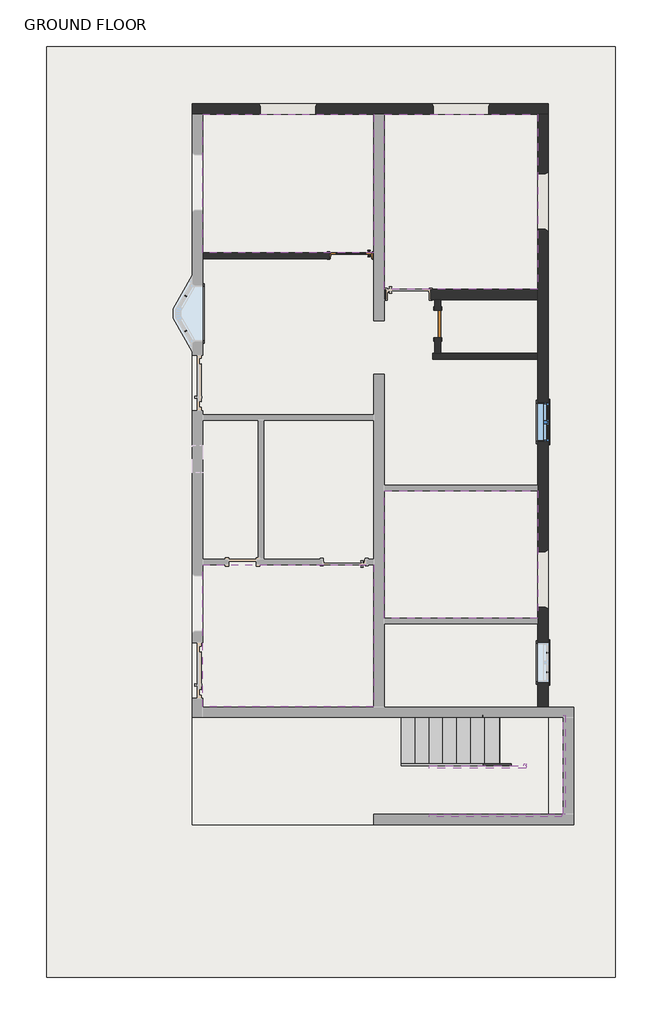
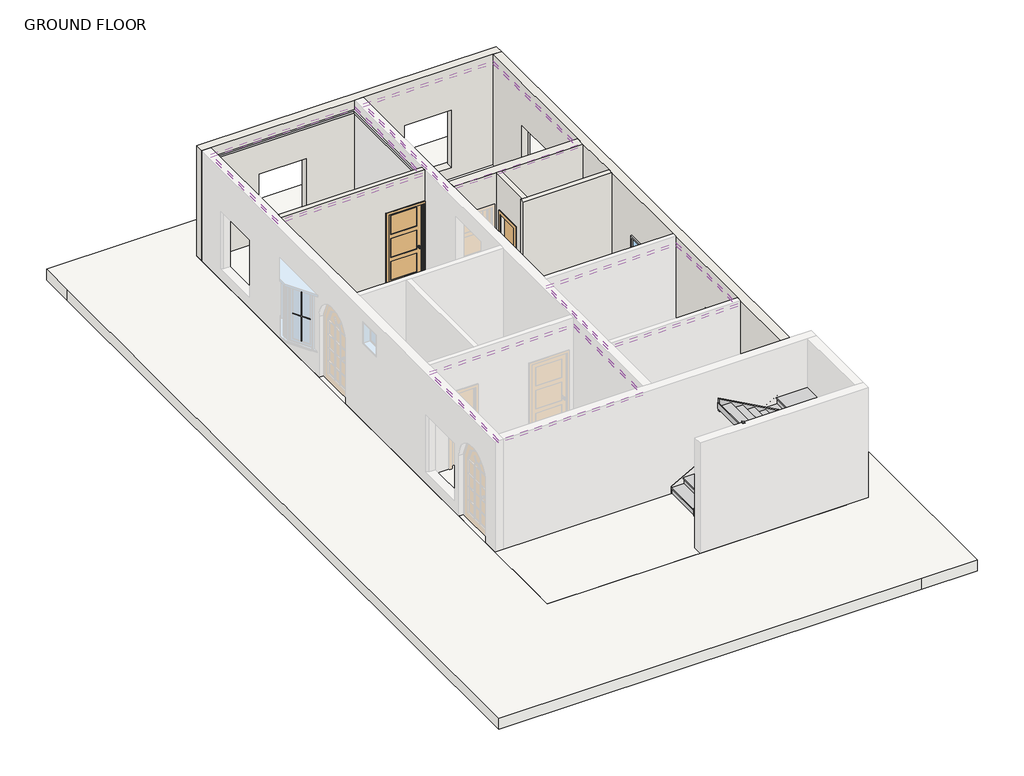
# One storey, part 2 of 2: 12 proxies, 8 coverings, 6 members, 6 walls, 2 doors, 2 slabs, 1 stair flight, 1 window.
"""IFC4 building model written with IfcOpenShell, lengths in millimetres."""

from ifc_helpers import new_model, si_unit, frame, origin, origin_with_axes, place, context, project, spatial, polyline, outline, extrude, faceted_brep, transform, mapped, element, save
from components import generic_models_1_generic_models_1_a1fc493f, muntin_pattern_2x2_muntin_pattern_2x2_75bf01dd, muntin_pattern_2x2_muntin_pattern_2x2_32baafd4, muntin_pattern_2x2_muntin_pattern_2x2_b3fe6957, muntin_pattern_2x2_muntin_pattern_2x2_3e0ecaf2, trim_window_exterior_flat_with_sill_41619996, trim_window_interior_flat_picture_frame_1060724f, trim_window_interior_flat_picture_frame_51c85655, door_b31adefa, single_flush_bathroom_flush_door_2_x_7_025d1c86, stair_flight_68498a3f, window_339605e1

model = new_model("IFC4")

# Units and contexts
model_context = context("Model", 3, world=origin())
ifc_project = project(units=[si_unit("LENGTHUNIT", "METRE", prefix="MILLI")], contexts=[model_context])

# Site, building, storey
site = spatial("IfcSite", under=ifc_project)
building = spatial("IfcBuilding", under=site)
storey = spatial("IfcBuildingStorey", under=building, Name="GROUND FLOOR", Elevation=304.8)

# Proxies
placement = place(None, origin())
generic_models_1_generic_models_1_shape = generic_models_1_generic_models_1_a1fc493f(model_context)
element("IfcBuildingElementProxy", 1, Name="Generic Models 1 : Generic Models 1", ObjectType="Generic Models 1 : Generic Models 1", at=placement, inside=storey, context=model_context, shape_type="MappedRepresentation", body=[
    mapped(generic_models_1_generic_models_1_shape, transform((0.0, 0.0, 0.0), x_axis=(1.0, 0.0, 0.0), y_axis=(0.0, 1.0, 0.0), z_axis=(0.0, 0.0, 1.0))),
])
muntin_pattern_2x2_muntin_pattern_2x2_shape = muntin_pattern_2x2_muntin_pattern_2x2_75bf01dd(model_context)
element("IfcBuildingElementProxy", 2, Name="Muntin Pattern_2x2 : Muntin Pattern_2x2", ObjectType="Muntin Pattern_2x2 : Muntin Pattern_2x2", at=placement, inside=storey, context=model_context, shape_type="MappedRepresentation", body=[
    mapped(muntin_pattern_2x2_muntin_pattern_2x2_shape, transform((-17494.1197687, 6617.7003691, 1035.05), x_axis=(-0.49999999999999245, 0.866025403784443, 0.0), y_axis=(-0.866025403784443, -0.49999999999999245, 0.0), z_axis=(0.0, 0.0, 1.0))),
])
muntin_pattern_2x2_muntin_pattern_2x2_2_shape = muntin_pattern_2x2_muntin_pattern_2x2_32baafd4(model_context)
element("IfcBuildingElementProxy", 3, Name="Muntin Pattern_2x2 : Muntin Pattern_2x2", ObjectType="Muntin Pattern_2x2 : Muntin Pattern_2x2", at=placement, inside=storey, context=model_context, shape_type="MappedRepresentation", body=[
    mapped(muntin_pattern_2x2_muntin_pattern_2x2_2_shape, transform((-17494.1197687, 7380.2948055, 1035.05), x_axis=(-0.4999999999999952, -0.8660254037844415, 0.0), y_axis=(0.8660254037844415, -0.4999999999999952, 0.0), z_axis=(0.0, 0.0, 1.0))),
])
muntin_pattern_2x2_muntin_pattern_2x2_3_shape = muntin_pattern_2x2_muntin_pattern_2x2_b3fe6957(model_context)
element("IfcBuildingElementProxy", 4, Name="Muntin Pattern_2x2 : Muntin Pattern_2x2", ObjectType="Muntin Pattern_2x2 : Muntin Pattern_2x2", at=placement, inside=storey, context=model_context, shape_type="MappedRepresentation", body=[
    mapped(muntin_pattern_2x2_muntin_pattern_2x2_3_shape, transform((-9539.4686606, -457.4899127, 1289.05), x_axis=(0.0, -1.0, 0.0), y_axis=(1.0, 0.0, 0.0), z_axis=(0.0, 0.0, 1.0))),
])
element("IfcBuildingElementProxy", 5, Name="Muntin Pattern_2x2 : Muntin Pattern_2x2", ObjectType="Muntin Pattern_2x2 : Muntin Pattern_2x2", at=placement, inside=storey, context=model_context, shape_type="MappedRepresentation", body=[
    mapped(muntin_pattern_2x2_muntin_pattern_2x2_3_shape, transform((-9539.4686606, 4825.7100873, 1289.05), x_axis=(0.0, -1.0, 0.0), y_axis=(1.0, 0.0, 0.0), z_axis=(0.0, 0.0, 1.0))),
])
muntin_pattern_2x2_muntin_pattern_2x2_4_shape = muntin_pattern_2x2_muntin_pattern_2x2_3e0ecaf2(model_context)
element("IfcBuildingElementProxy", 6, Name="Muntin Pattern_2x2 : Muntin Pattern_2x2", ObjectType="Muntin Pattern_2x2 : Muntin Pattern_2x2", at=placement, inside=storey, context=model_context, shape_type="MappedRepresentation", body=[
    mapped(muntin_pattern_2x2_muntin_pattern_2x2_4_shape, transform((-9539.4686606, -886.1149127, 1289.05), x_axis=(0.0, 1.0, 0.0), y_axis=(-1.0, 0.0, 0.0), z_axis=(0.0, 0.0, 1.0))),
])
element("IfcBuildingElementProxy", 7, Name="Muntin Pattern_2x2 : Muntin Pattern_2x2", ObjectType="Muntin Pattern_2x2 : Muntin Pattern_2x2", at=placement, inside=storey, context=model_context, shape_type="MappedRepresentation", body=[
    mapped(muntin_pattern_2x2_muntin_pattern_2x2_4_shape, transform((-9539.4686606, 4397.0850873, 1289.05), x_axis=(0.0, 1.0, 0.0), y_axis=(-1.0, 0.0, 0.0), z_axis=(0.0, 0.0, 1.0))),
])
trim_window_exterior_flat_with_sill_shape = trim_window_exterior_flat_with_sill_41619996(model_context)
element("IfcBuildingElementProxy", 8, Name="Trim-Window-Exterior-Flat : with Sill", ObjectType="Trim-Window-Exterior-Flat : with Sill", at=placement, inside=storey, context=model_context, shape_type="MappedRepresentation", body=[
    mapped(trim_window_exterior_flat_with_sill_shape, transform((-9529.9436606, -671.8024127, 2133.6), x_axis=(0.0, 1.0, 0.0), y_axis=(0.0, 0.0, 1.0), z_axis=(1.0, 0.0, 0.0))),
])
element("IfcBuildingElementProxy", 9, Name="Trim-Window-Exterior-Flat : with Sill", ObjectType="Trim-Window-Exterior-Flat : with Sill", at=placement, inside=storey, context=model_context, shape_type="MappedRepresentation", body=[
    mapped(trim_window_exterior_flat_with_sill_shape, transform((-9529.9436606, 4611.3975873, 2133.6), x_axis=(0.0, 1.0, 0.0), y_axis=(0.0, 0.0, 1.0), z_axis=(1.0, 0.0, 0.0))),
])
trim_window_interior_flat_picture_frame_shape = trim_window_interior_flat_picture_frame_1060724f(model_context)
element("IfcBuildingElementProxy", 10, Name="Trim-Window-Interior-Flat : Picture Frame", ObjectType="Trim-Window-Interior-Flat : Picture Frame", at=placement, inside=storey, context=model_context, shape_type="MappedRepresentation", body=[
    mapped(trim_window_interior_flat_picture_frame_shape, transform((-17124.5436606, 6998.9975873, 2489.2), x_axis=(0.0, 1.0, 0.0), y_axis=(0.0, 0.0, 1.0), z_axis=(1.0, 0.0, 0.0))),
])
trim_window_interior_flat_picture_frame_2_shape = trim_window_interior_flat_picture_frame_51c85655(model_context)
element("IfcBuildingElementProxy", 11, Name="Trim-Window-Interior-Flat : Picture Frame", ObjectType="Trim-Window-Interior-Flat : Picture Frame", at=placement, inside=storey, context=model_context, shape_type="MappedRepresentation", body=[
    mapped(trim_window_interior_flat_picture_frame_2_shape, transform((-9758.5436606, -671.8024127, 2133.6), x_axis=(0.0, -1.0, 0.0), y_axis=(0.0, 0.0, 1.0), z_axis=(-1.0, 0.0, 0.0))),
])
element("IfcBuildingElementProxy", 12, Name="Trim-Window-Interior-Flat : Picture Frame", ObjectType="Trim-Window-Interior-Flat : Picture Frame", at=placement, inside=storey, context=model_context, shape_type="MappedRepresentation", body=[
    mapped(trim_window_interior_flat_picture_frame_2_shape, transform((-9758.5436606, 4611.3975873, 2133.6), x_axis=(0.0, -1.0, 0.0), y_axis=(0.0, 0.0, 1.0), z_axis=(-1.0, 0.0, 0.0))),
])

# Coverings
element("IfcCovering", 13, ObjectType="ceiling", at=placement, inside=storey, context=model_context, shape_type="SweptSolid", body=[
    extrude(outline(polyline([(-17124.5436606, 8332.4975873), (-17124.5436606, 11380.4975873), (-13365.3436606, 11380.4975873), (-13365.3436606, 8332.4975873), (-17124.5436606, 8332.4975873)])), frame((0.0, 0.0, 3175.0), z_axis=(0.0, 0.0, 1.0), x_axis=(1.0, 0.0, 0.0)), (0.0, 0.0, 1.0), 107.95),
])
element("IfcCovering", 14, ObjectType="ceiling", at=placement, inside=storey, context=model_context, shape_type="SweptSolid", body=[
    extrude(outline(polyline([(-13365.3436606, 11380.4975873), (-13365.3436606, 8332.4975873), (-17124.5436606, 8332.4975873), (-17124.5436606, 11380.4975873), (-13365.3436606, 11380.4975873)]), holes=[polyline([(-13670.1436606, 11075.6975873), (-16819.7436606, 11075.6975873), (-16819.7436606, 8637.2975873), (-13670.1436606, 8637.2975873), (-13670.1436606, 11075.6975873)])]), frame((0.0, 0.0, 3098.8), z_axis=(0.0, 0.0, 1.0), x_axis=(1.0, 0.0, 0.0)), (0.0, 0.0, 1.0), 107.95),
    extrude(outline(polyline([(-14279.7436606, 10466.0975873), (-14279.7436606, 9246.8975873), (-16210.1436606, 9246.8975873), (-16210.1436606, 10466.0975873), (-14279.7436606, 10466.0975873)])), frame((0.0, 0.0, 3098.8), z_axis=(0.0, 0.0, 1.0), x_axis=(1.0, 0.0, 0.0)), (0.0, 0.0, 1.0), 107.95),
])
element("IfcCovering", 15, ObjectType="ceiling", at=placement, inside=storey, context=model_context, shape_type="SweptSolid", body=[
    extrude(outline(polyline([(-13136.7436606, 7532.3975873), (-13136.7436606, 11380.4975873), (-9758.5436606, 11380.4975873), (-9758.5436606, 7532.3975873), (-13136.7436606, 7532.3975873)])), frame((0.0, 0.0, 3175.0), z_axis=(0.0, 0.0, 1.0), x_axis=(1.0, 0.0, 0.0)), (0.0, 0.0, 1.0), 107.95),
])
element("IfcCovering", 16, ObjectType="ceiling", at=placement, inside=storey, context=model_context, shape_type="SweptSolid", body=[
    extrude(outline(polyline([(-9758.5436606, 11380.4975873), (-9758.5436606, 7532.3975873), (-13136.7436606, 7532.3975873), (-13136.7436606, 11380.4975873), (-9758.5436606, 11380.4975873)]), holes=[polyline([(-10063.3436606, 11075.6975873), (-12831.9436606, 11075.6975873), (-12831.9436606, 7837.1975873), (-10063.3436606, 7837.1975873), (-10063.3436606, 11075.6975873)])]), frame((0.0, 0.0, 3098.8), z_axis=(0.0, 0.0, 1.0), x_axis=(1.0, 0.0, 0.0)), (0.0, 0.0, 1.0), 107.95),
    extrude(outline(polyline([(-10672.9436606, 10466.0975873), (-10672.9436606, 8446.7975873), (-12222.3436606, 8446.7975873), (-12222.3436606, 10466.0975873), (-10672.9436606, 10466.0975873)])), frame((0.0, 0.0, 3098.8), z_axis=(0.0, 0.0, 1.0), x_axis=(1.0, 0.0, 0.0)), (0.0, 0.0, 1.0), 107.95),
])
element("IfcCovering", 17, ObjectType="ceiling", at=placement, inside=storey, context=model_context, shape_type="SweptSolid", body=[
    extrude(outline(polyline([(-13365.3436606, -1649.7024127), (-17124.5436606, -1649.7024127), (-17124.5436606, 1474.4975873), (-13365.3436606, 1474.4975873), (-13365.3436606, -1649.7024127)])), frame((0.0, 0.0, 3175.0), z_axis=(0.0, 0.0, 1.0), x_axis=(1.0, 0.0, 0.0)), (0.0, 0.0, 1.0), 107.95),
])
element("IfcCovering", 18, ObjectType="ceiling", at=placement, inside=storey, context=model_context, shape_type="SweptSolid", body=[
    extrude(outline(polyline([(-13365.3436606, 1474.4975873), (-13365.3436606, -1649.7024127), (-17124.5436606, -1649.7024127), (-17124.5436606, 1474.4975873), (-13365.3436606, 1474.4975873)]), holes=[polyline([(-13670.1436606, 1169.6975873), (-16819.7436606, 1169.6975873), (-16819.7436606, -1344.9024127), (-13670.1436606, -1344.9024127), (-13670.1436606, 1169.6975873)])]), frame((0.0, 0.0, 3098.8), z_axis=(0.0, 0.0, 1.0), x_axis=(1.0, 0.0, 0.0)), (0.0, 0.0, 1.0), 107.95),
    extrude(outline(polyline([(-14279.7436606, 560.0975873), (-14279.7436606, -735.3024127), (-16210.1436606, -735.3024127), (-16210.1436606, 560.0975873), (-14279.7436606, 560.0975873)])), frame((0.0, 0.0, 3098.8), z_axis=(0.0, 0.0, 1.0), x_axis=(1.0, 0.0, 0.0)), (0.0, 0.0, 1.0), 107.95),
])
element("IfcCovering", 19, ObjectType="ceiling", at=placement, inside=storey, context=model_context, shape_type="SweptSolid", body=[
    extrude(outline(polyline([(-9758.5436606, 3100.0975873), (-9758.5436606, 306.0975873), (-13136.7436606, 306.0975873), (-13136.7436606, 3100.0975873), (-9758.5436606, 3100.0975873)])), frame((0.0, 0.0, 3175.0), z_axis=(0.0, 0.0, 1.0), x_axis=(1.0, 0.0, 0.0)), (0.0, 0.0, 1.0), 107.95),
])
element("IfcCovering", 20, ObjectType="ceiling", at=placement, inside=storey, context=model_context, shape_type="SweptSolid", body=[
    extrude(outline(polyline([(-9758.5436606, 3100.0975873), (-9758.5436606, 306.0975873), (-13136.7436606, 306.0975873), (-13136.7436606, 3100.0975873), (-9758.5436606, 3100.0975873)]), holes=[polyline([(-10063.3436606, 2795.2975873), (-12831.9436606, 2795.2975873), (-12831.9436606, 610.8975873), (-10063.3436606, 610.8975873), (-10063.3436606, 2795.2975873)])]), frame((0.0, 0.0, 3098.8), z_axis=(0.0, 0.0, 1.0), x_axis=(1.0, 0.0, 0.0)), (0.0, 0.0, 1.0), 107.95),
    extrude(outline(polyline([(-10672.9436606, 2185.6975873), (-10672.9436606, 1220.4975873), (-12222.3436606, 1220.4975873), (-12222.3436606, 2185.6975873), (-10672.9436606, 2185.6975873)])), frame((0.0, 0.0, 3098.8), z_axis=(0.0, 0.0, 1.0), x_axis=(1.0, 0.0, 0.0)), (0.0, 0.0, 1.0), 107.95),
])

# Doors
door_shape = door_b31adefa(model_context)
element("IfcDoor", 21, ObjectType="Door-Interior-Single-3_Panel_Vert-Wood : 36\" x 84\"", at=placement, inside=storey, context=model_context, shape_type="MappedRepresentation", body=[
    mapped(door_shape, transform((-13860.6436606, 8272.1725873, 304.8), x_axis=(-1.0, 0.0, 0.0), y_axis=(0.0, -1.0, 0.0), z_axis=(0.0, 0.0, 1.0))),
])
single_flush_bathroom_flush_door_2_x_7_shape = single_flush_bathroom_flush_door_2_x_7_025d1c86(model_context)
element("IfcDoor", 22, ObjectType="Single-Flush : BATHROOM FLUSH DOOR 2' X 7'", at=placement, inside=storey, context=model_context, shape_type="MappedRepresentation", body=[
    mapped(single_flush_bathroom_flush_door_2_x_7_shape, transform((-11955.6436606, 6770.3975873, 304.8), x_axis=(0.0, -1.0, 0.0), y_axis=(1.0, 0.0, 0.0), z_axis=(0.0, 0.0, 1.0))),
])

# Members
element("IfcMember", 23, ObjectType="Stringer - 2\" Width", at=placement, inside=storey, context=model_context, shape_type="SweptSolid", body=[
    extrude(outline(polyline([(512.3983948, -12755.7436606), (304.8, -12755.7436606), (304.8, -12501.7991578), (2074.3333333, -9316.6391578), (2074.3333333, -9944.2607712), (512.3983948, -12755.7436606)])), frame((0.0, -1878.3024127, 0.0), z_axis=(0.0, 1.0, 0.0), x_axis=(0.0, 0.0, 1.0)), (0.0, 0.0, 1.0), 50.8),
])
element("IfcMember", 24, ObjectType="Stringer - 2\" Width", at=placement, inside=storey, context=model_context, shape_type="SweptSolid", body=[
    extrude(outline(polyline([(-9199.7436606, -1827.5024127), (-9148.9436606, -1827.5024127), (-9148.9436606, -4011.9024127), (-9199.7436606, -4011.9024127), (-9199.7436606, -1827.5024127)])), frame((0.0, 0.0, 1769.5333333), z_axis=(0.0, 0.0, 1.0), x_axis=(1.0, 0.0, 0.0)), (0.0, 0.0, 1.0), 304.8),
])
element("IfcMember", 25, ObjectType="Stringer - 2\" Width", at=placement, inside=storey, context=model_context, shape_type="SweptSolid", body=[
    extrude(outline(polyline([(1769.5333333, -9227.38655), (3391.0650614, -12146.1436606), (3042.3863873, -12146.1436606), (1769.5333333, -9855.0081634), (1769.5333333, -9227.38655)])), frame((0.0, -4062.7024127, 0.0), z_axis=(0.0, 1.0, 0.0), x_axis=(0.0, 0.0, 1.0)), (0.0, 0.0, 1.0), 50.8),
])
element("IfcMember", 26, ObjectType="Stringer - 2\" Width", at=placement, inside=storey, context=model_context, shape_type="SweptSolid", body=[
    extrude(outline(polyline([(512.3983948, -12755.7436606), (304.8, -12755.7436606), (304.8, -12501.7991578), (1659.4974984, -10063.3436606), (2008.1761726, -10063.3436606), (512.3983948, -12755.7436606)])), frame((0.0, -2945.1024127, 0.0), z_axis=(0.0, 1.0, 0.0), x_axis=(0.0, 0.0, 1.0)), (0.0, 0.0, 1.0), 50.8),
])
element("IfcMember", 27, ObjectType="Stringer - 2\" Width", at=placement, inside=storey, context=model_context, shape_type="SweptSolid", body=[
    extrude(outline(polyline([(-10063.3436606, -2894.3024127), (-10012.5436606, -2894.3024127), (-10012.5436606, -2945.1024127), (-10063.3436606, -2945.1024127), (-10063.3436606, -2894.3024127)])), frame((0.0, 0.0, 1769.5333333), z_axis=(0.0, 0.0, 1.0), x_axis=(1.0, 0.0, 0.0)), (0.0, 0.0, 1.0), 304.8),
])
element("IfcMember", 28, ObjectType="Stringer - 2\" Width", at=placement, inside=storey, context=model_context, shape_type="SweptSolid", body=[
    extrude(outline(polyline([(1857.053054, -10012.5436606), (2205.7317281, -10012.5436606), (3391.0650614, -12146.1436606), (3042.3863873, -12146.1436606), (1857.053054, -10012.5436606)])), frame((0.0, -2995.9024127, 0.0), z_axis=(0.0, 1.0, 0.0), x_axis=(0.0, 0.0, 1.0)), (0.0, 0.0, 1.0), 50.8),
])

# Slabs
element("IfcSlab", 29, ObjectType="MARBLE FLOORING 1'", at=placement, inside=storey, context=model_context, shape_type="SweptSolid", body=[
    extrude(outline(polyline([(-9529.9436606, 11609.0975873), (-9529.9436606, -4240.5024127), (-17353.1436606, -4240.5024127), (-17353.1436606, 11609.0975873), (-9529.9436606, 11609.0975873)])), origin_with_axes(), (0.0, 0.0, 1.0), 304.8),
])
element("IfcSlab", 30, ObjectType="VERANDA FLOORING", at=placement, inside=storey, context=model_context, shape_type="SweptSolid", body=[
    extrude(outline(polyline([(-20553.5436606, -7593.3024127), (-20553.5436606, 11926.5975873), (-20553.5436606, 12866.3975873), (-8056.7436606, 12866.3975873), (-8056.7436606, -7593.3024127), (-9529.9436606, -7593.3024127), (-20553.5436606, -7593.3024127)]), holes=[polyline([(-17353.1436606, -4240.5024127), (-9529.9436606, -4240.5024127), (-9529.9436606, -1649.7024127), (-9529.9436606, 11609.0975873), (-17353.1436606, 11609.0975873), (-17353.1436606, -4240.5024127)])]), origin_with_axes(), (0.0, 0.0, 1.0), 304.8),
])

# Stair flight
stair_flight_shape = stair_flight_68498a3f(model_context)
element("IfcStairFlight", 31, ObjectType="2\" Tread 1\" Nosing 1/4\" Riser", at=placement, inside=storey, context=model_context, shape_type="MappedRepresentation", body=[
    mapped(stair_flight_shape, transform((0.0, 0.0, 0.0), x_axis=(1.0, 0.0, 0.0), y_axis=(0.0, 1.0, 0.0), z_axis=(0.0, 0.0, 1.0))),
])

# Walls
element("IfcWall", 32, at=placement, inside=storey, context=model_context, shape_type="Brep", body=[
    faceted_brep([(-17353.1436606, 11380.4975873, 304.8), (-17124.5436606, 11380.4975873, 304.8), (-13365.3436606, 11380.4975873, 304.8), (-13136.7436606, 11380.4975873, 304.8), (-9758.5436606, 11380.4975873, 304.8), (-9529.9436606, 11380.4975873, 304.8), (-9529.9436606, 11380.4975873, 3352.8), (-9758.5436606, 11380.4975873, 3352.8), (-13136.7436606, 11380.4975873, 3352.8), (-13365.3436606, 11380.4975873, 3352.8), (-17124.5436606, 11380.4975873, 3352.8), (-17353.1436606, 11380.4975873, 3352.8), (-15854.5436606, 11380.4975873, 2184.4), (-14635.3436606, 11380.4975873, 2184.4), (-14635.3436606, 11380.4975873, 609.6), (-15854.5436606, 11380.4975873, 609.6), (-12057.2436606, 11380.4975873, 2184.4), (-10838.0436606, 11380.4975873, 2184.4), (-10838.0436606, 11380.4975873, 609.6), (-12057.2436606, 11380.4975873, 609.6), (-17353.1436606, 11609.0975873, 304.8), (-17353.1436606, 11609.0975873, 3352.8), (-9529.9436606, 11609.0975873, 3352.8), (-9529.9436606, 11609.0975873, 304.8), (-14600.4186606, 11609.0975873, 2184.4), (-15889.4686606, 11609.0975873, 2184.4), (-15889.4686606, 11609.0975873, 609.6), (-14600.4186606, 11609.0975873, 609.6), (-10803.1186606, 11609.0975873, 2184.4), (-12092.1686606, 11609.0975873, 2184.4), (-12092.1686606, 11609.0975873, 609.6), (-10803.1186606, 11609.0975873, 609.6), (-15854.5436606, 11548.6057128, 2184.4), (-14635.3436606, 11548.6057128, 2184.4), (-15854.5436606, 11548.6057128, 609.6), (-14635.3436606, 11548.6057128, 609.6), (-12057.2436606, 11548.6057128, 2184.4), (-10838.0436606, 11548.6057128, 2184.4), (-12057.2436606, 11548.6057128, 609.6), (-10838.0436606, 11548.6057128, 609.6)], [[[0, 1, 2, 3, 4, 5, 6, 7, 8, 9, 10, 11], [12, 13, 14, 15], [16, 17, 18, 19]], [[20, 21, 22, 23], [24, 25, 26, 27], [28, 29, 30, 31]], [[5, 4, 3, 2, 1, 0, 20, 23]], [[11, 10, 9, 8, 7, 6, 22, 21]], [[0, 11, 21, 20]], [[6, 5, 23, 22]], [[32, 25, 24, 33, 13, 12]], [[34, 15, 14, 35, 27, 26]], [[32, 12, 15, 34]], [[13, 33, 35, 14]], [[33, 24, 27, 35]], [[25, 32, 34, 26]], [[36, 29, 28, 37, 17, 16]], [[38, 19, 18, 39, 31, 30]], [[36, 16, 19, 38]], [[17, 37, 39, 18]], [[37, 28, 31, 39]], [[29, 36, 38, 30]]]),
])
element("IfcWall", 33, at=placement, inside=storey, context=model_context, shape_type="Brep", body=[
    faceted_brep([(-9529.9436606, -1649.7024127, 304.8), (-9529.9436606, 11380.4975873, 304.8), (-9529.9436606, 11380.4975873, 3352.8), (-9529.9436606, -1649.7024127, 3352.8), (-9529.9436606, 8811.9225873, 2184.4), (-9529.9436606, 10100.9725873, 2184.4), (-9529.9436606, 10100.9725873, 609.6), (-9529.9436606, 8811.9225873, 609.6), (-9529.9436606, 512.4725873, 2184.4), (-9529.9436606, 1801.5225873, 2184.4), (-9529.9436606, 1801.5225873, 609.6), (-9529.9436606, 512.4725873, 609.6), (-9529.9436606, -1103.6024127, 2133.6), (-9529.9436606, -240.0024127, 2133.6), (-9529.9436606, -240.0024127, 1219.2), (-9529.9436606, -1103.6024127, 1219.2), (-9529.9436606, 4179.5975873, 2133.6), (-9529.9436606, 5043.1975873, 2133.6), (-9529.9436606, 5043.1975873, 1219.2), (-9529.9436606, 4179.5975873, 1219.2), (-9758.5436606, -1649.7024127, 304.8), (-9758.5436606, -1649.7024127, 3352.8), (-9758.5436606, 179.0975873, 3352.8), (-9758.5436606, 306.0975873, 3352.8), (-9758.5436606, 3100.0975873, 3352.8), (-9758.5436606, 3227.0975873, 3352.8), (-9758.5436606, 5995.6975873, 3352.8), (-9758.5436606, 6122.6975873, 3352.8), (-9758.5436606, 7303.7975873, 3352.8), (-9758.5436606, 7532.3975873, 3352.8), (-9758.5436606, 11380.4975873, 3352.8), (-9758.5436606, 11380.4975873, 304.8), (-9758.5436606, 7532.3975873, 304.8), (-9758.5436606, 7303.7975873, 304.8), (-9758.5436606, 6122.6975873, 304.8), (-9758.5436606, 5995.6975873, 304.8), (-9758.5436606, 3227.0975873, 304.8), (-9758.5436606, 3100.0975873, 304.8), (-9758.5436606, 306.0975873, 304.8), (-9758.5436606, 179.0975873, 304.8), (-9758.5436606, 10066.0475873, 2184.4), (-9758.5436606, 8846.8475873, 2184.4), (-9758.5436606, 8846.8475873, 609.6), (-9758.5436606, 10066.0475873, 609.6), (-9758.5436606, 1766.5975873, 2184.4), (-9758.5436606, 547.3975873, 2184.4), (-9758.5436606, 547.3975873, 609.6), (-9758.5436606, 1766.5975873, 609.6), (-9758.5436606, -1103.6024127, 2133.6), (-9758.5436606, -1103.6024127, 1219.2), (-9758.5436606, -240.0024127, 1219.2), (-9758.5436606, -240.0024127, 2133.6), (-9758.5436606, 4179.5975873, 2133.6), (-9758.5436606, 4179.5975873, 1219.2), (-9758.5436606, 5043.1975873, 1219.2), (-9758.5436606, 5043.1975873, 2133.6), (-9590.4355351, 10066.0475873, 2184.4), (-9590.4355351, 8846.8475873, 2184.4), (-9590.4355351, 10066.0475873, 609.6), (-9590.4355351, 8846.8475873, 609.6), (-9590.4355351, 1766.5975873, 2184.4), (-9590.4355351, 547.3975873, 2184.4), (-9590.4355351, 1766.5975873, 609.6), (-9590.4355351, 547.3975873, 609.6)], [[[0, 1, 2, 3], [4, 5, 6, 7], [8, 9, 10, 11], [12, 13, 14, 15], [16, 17, 18, 19]], [[20, 21, 22, 23, 24, 25, 26, 27, 28, 29, 30, 31, 32, 33, 34, 35, 36, 37, 38, 39], [40, 41, 42, 43], [44, 45, 46, 47], [48, 49, 50, 51], [52, 53, 54, 55]], [[1, 0, 20, 39, 38, 37, 36, 35, 34, 33, 32, 31]], [[3, 2, 30, 29, 28, 27, 26, 25, 24, 23, 22, 21]], [[2, 1, 31, 30]], [[0, 3, 21, 20]], [[56, 5, 4, 57, 41, 40]], [[58, 43, 42, 59, 7, 6]], [[56, 40, 43, 58]], [[41, 57, 59, 42]], [[57, 4, 7, 59]], [[5, 56, 58, 6]], [[60, 9, 8, 61, 45, 44]], [[62, 47, 46, 63, 11, 10]], [[60, 44, 47, 62]], [[45, 61, 63, 46]], [[61, 8, 11, 63]], [[9, 60, 62, 10]], [[49, 48, 12, 15]], [[50, 49, 15, 14]], [[51, 50, 14, 13]], [[48, 51, 13, 12]], [[53, 52, 16, 19]], [[54, 53, 19, 18]], [[55, 54, 18, 17]], [[52, 55, 17, 16]]]),
])
element("IfcWall", 34, at=placement, inside=storey, context=model_context, shape_type="Brep", body=[
    faceted_brep([(-13136.7436606, 7532.3975873, 3352.8), (-9758.5436606, 7532.3975873, 3352.8), (-9758.5436606, 7532.3975873, 304.8), (-12120.7436606, 7532.3975873, 304.8), (-12120.7436606, 7532.3975873, 2463.8), (-13085.9436606, 7532.3975873, 2463.8), (-13085.9436606, 7532.3975873, 304.8), (-13136.7436606, 7532.3975873, 304.8), (-9758.5436606, 7303.7975873, 3352.8), (-11892.1436606, 7303.7975873, 3352.8), (-12019.1436606, 7303.7975873, 3352.8), (-13136.7436606, 7303.7975873, 3352.8), (-13136.7436606, 7303.7975873, 304.8), (-13085.9436606, 7303.7975873, 304.8), (-13085.9436606, 7303.7975873, 2463.8), (-12120.7436606, 7303.7975873, 2463.8), (-12120.7436606, 7303.7975873, 304.8), (-12019.1436606, 7303.7975873, 304.8), (-11892.1436606, 7303.7975873, 304.8), (-9758.5436606, 7303.7975873, 304.8)], [[[0, 1, 2, 3, 4, 5, 6, 7]], [[8, 9, 10, 11, 12, 13, 14, 15, 16, 17, 18, 19]], [[2, 19, 18, 17, 16, 3]], [[12, 7, 6, 13]], [[1, 0, 11, 10, 9, 8]], [[2, 1, 8, 19]], [[0, 7, 12, 11]], [[15, 4, 3, 16]], [[4, 15, 14, 5]], [[5, 14, 13, 6]]]),
])
element("IfcWall", 35, ObjectType="INNER WALL 5\"", at=placement, inside=storey, context=model_context, shape_type="SweptSolid", body=[
    extrude(outline(polyline([(3352.8, -13365.3436606), (3352.8, -17124.5436606), (304.8, -17124.5436606), (304.8, -14343.2436606), (2463.8, -14343.2436606), (2463.8, -13378.0436606), (304.8, -13378.0436606), (304.8, -13365.3436606), (3352.8, -13365.3436606)])), frame((0.0, 8205.4975873, 0.0), z_axis=(0.0, 1.0, 0.0), x_axis=(0.0, 0.0, 1.0)), (0.0, 0.0, 1.0), 127.0),
])
element("IfcWall", 36, ObjectType="INNER WALL 5\"", at=placement, inside=storey, context=model_context, shape_type="Brep", body=[
    faceted_brep([(-9758.5436606, 6122.6975873, 304.8), (-11892.1436606, 6122.6975873, 304.8), (-12019.1436606, 6122.6975873, 304.8), (-12069.9436606, 6122.6975873, 304.8), (-12069.9436606, 6122.6975873, 3352.8), (-12019.1436606, 6122.6975873, 3352.8), (-11892.1436606, 6122.6975873, 3352.8), (-9758.5436606, 6122.6975873, 3352.8), (-9758.5436606, 5995.6975873, 304.8), (-9758.5436606, 5995.6975873, 3352.8), (-12069.9436606, 5995.6975873, 3352.8), (-12069.9436606, 5995.6975873, 304.8)], [[[0, 1, 2, 3, 4, 5, 6, 7]], [[8, 9, 10, 11]], [[3, 2, 1, 0, 8, 11]], [[4, 3, 11, 10]], [[7, 6, 5, 4, 10, 9]], [[0, 7, 9, 8]]]),
])
element("IfcWall", 37, ObjectType="INNER WALL 5\"", at=placement, inside=storey, context=model_context, shape_type="SweptSolid", body=[
    extrude(outline(polyline([(6122.6975873, 3352.8), (7303.7975873, 3352.8), (7303.7975873, 304.8), (7075.1975873, 304.8), (7075.1975873, 2336.8), (6465.5975873, 2336.8), (6465.5975873, 304.8), (6122.6975873, 304.8), (6122.6975873, 3352.8)])), frame((-12019.1436606, 0.0, 0.0), z_axis=(1.0, 0.0, 0.0), x_axis=(0.0, 1.0, 0.0)), (0.0, 0.0, 1.0), 127.0),
])

# Window
window_shape = window_339605e1(model_context)
element("IfcWindow", 38, ObjectType="Window-Casement-Double : 34\" x 36\"", at=placement, inside=storey, context=model_context, shape_type="MappedRepresentation", body=[
    mapped(window_shape, transform((-9644.2436606, 4611.3975873, 304.8), x_axis=(0.0, -1.0, 0.0), y_axis=(1.0, 0.0, 0.0), z_axis=(0.0, 0.0, 1.0))),
])

save(model, "model.ifc")

# Revit data of these elements
# Type "Muntin Pattern_2x2 : Muntin Pattern_2x2"
#   Width [instance default] = 4' - 0"
#   Thickness = 0' - 0 1/2"
#   Height [instance default] = 4' - 0"
#   Distance = 0' - 0 3/4"
#   Interior Material [instance default] = none
#   Exterior Material [instance default] = none
#   Default Elevation = 0
# Type "Trim-Window-Exterior-Flat : with Sill"
#   Trim Width = 0' - 2 1/4"
#   Trim Thickness_Picture Frame = 0' - 1 1/4"
#   Trim Thickness_with Sill = 0' - 0 3/4"
#   Sill Thickness = 0' - 1 1/4"
#   Opening Width [instance default] = 2' - 0"
#   Opening Height [instance default] = 3' - 0"
#   Default Elevation = 4' - 0"
#   Sill = yes
#   Picture Frame = no
#   Trim Material [instance default] = none
# Type "Trim-Window-Interior-Flat : Picture Frame"
#   Trim Thickness_Picture Frame = 0' - 1 1/4"
#   Trim Width = 0' - 2 1/4"
#   Trim Thickness_with Sill = 0' - 0 3/4"
#   Sill Thickness = 0' - 1 1/4"
#   Opening Width [instance default] = 2' - 0"
#   Opening Height [instance default] = 3' - 0"
#   Default Elevation = 4' - 0"
#   Sill = no
#   Picture Frame = yes
#   Trim Material [instance default] = none
# Type "ceiling"
#   Assembly Code = "C3030220"
#   built-in parameter 1002203 = 1 (stored number, unit not read)
#   built-in parameter 1002202 = 1 (stored number, unit not read)
#   Layers, outside or top first: 0' - 3 5/8" "Metal Stud Layer" (function 1); 0' - 0 5/8" "Gypsum Wall Board" (function 5)
# Type "Door-Interior-Single-3_Panel_Vert-Wood : 36\" x 84\""
#   Type Mark = "9"
#   Assembly Code = "C1020300"
#   Analytic Construction = "Wooden"
#   Top Rail = 0' - 4 11/16"
#   Thickness = 0' - 1 3/8"
#   Thermal Resistance (R) = 2.5876 (h·ft²·°F)/BTU
#   Swing Angle [instance default] = 90.00°
#   Stiles = 0' - 4 3/4"
#   Rough Width = 3' - 2"
#   Rough Height = 7' - 1"
#   Intermediate Rail = 0' - 4 1/2"
#   Height = 7' - 0"
#   Width = 3' - 0"
#   Heat Transfer Coefficient (U) = 0.3865 BTU/(h·ft²·°F)
#   Bottom Rail = 0' - 9 1/8"
#   Trim Material = Cherry
#   Panel Material = Cherry
#   Frame Material = Cherry
#   Door Handle Material = Aluminum
#   Visual Light Transmittance = 0
#   Solar Heat Gain Coefficient = 0
#   Wall Closure = (empty or 0)
#   Function = (empty or 0)
# Type "Single-Flush : BATHROOM FLUSH DOOR 2' X 7'"
#   Type Mark = "8"
#   Construction Type Id = "MDOOR"
#   Assembly Code = "C1020"
#   Analytic Construction = "Metal"
#   Thickness = 0' - 2"
#   Heat Transfer Coefficient (U) = 0.651978 BTU/(h·ft²·°F)
#   Height = 6' - 8"
#   Trim Projection Ext = 0' - 1"
#   Trim Projection Int = 0' - 1"
#   Trim Width = 0' - 3"
#   Width = 2' - 0"
#   Define Thermal Properties by = 1
#   Door Material = Door - Panel
#   Frame Material = Door - Frame
#   Visual Light Transmittance = 0
#   Solar Heat Gain Coefficient = 0
#   Function = (empty or 0)
#   Wall Closure = (empty or 0)
# Type "MARBLE FLOORING 1'"
#   Assembly Code = "B1010"
#   Function = 0
#   Layers, outside or top first: 1' - 0" "MARBLE FLOORING CLASSIC" (function 1)
# Type "VERANDA FLOORING"
#   Assembly Code = "B1010"
#   Function = 0
#   Layers, outside or top first: 1' - 0" "VERANDA AREA TILES" (function 1)
# Type
#   Assembly Code = "B2010"
#   Layers, outside or top first: 0' - 9" "TERRACOTTA" (function 1)
# Type "INNER WALL 5\""
#   Assembly Code = "B2010"
#   Layers, outside or top first: 0' - 5" "TERRACOTTA" (function 1)
# Type "Window-Casement-Double : 34\" x 36\""
#   Type Mark = "14"
#   Fire Rating = "0.5h"
#   Assembly Code = "B2020100"
#   Analytic Construction = "Double glazing - domestic"
#   Frame Extension [instance default] = 0' - 0 1/4"
#   Window Inset [instance default] = 0' - 0"
#   Wall Thickness [instance default] = 0' - 6"
#   Interior Wall Closure [instance default] = 0' - 2 1/4"
#   Half Width = 1' - 5"
#   Visual Light Transmittance = 0.81
#   Thermal Resistance (R) = 1.8146 (h·ft²·°F)/BTU
#   Solar Heat Gain Coefficient = 0.76
#   Rough Width = 2' - 10 1/2"
#   Rough Height = 3' - 0 1/2"
#   Height = 3' - 0"
#   Heat Transfer Coefficient (U) = 0.5511 BTU/(h·ft²·°F)
#   Exterior Wall Closure [instance default] = 0' - 1 1/4"
#   Extension Jamb [instance default] = 0' - 2 1/4"
#   Default Sill Height = 3' - 0"
#   Width = 2' - 10"
#   Define Thermal Properties by = 0
#   Muntin Visibility = yes
#   Interior Trim Visibility [instance default] = yes
#   Exterior Trim Visibility [instance default] = yes
#   Extension Jamb Visibility [instance default] = yes
#   Interior Trim Material = Wood - Stained
#   Muntin Pattern = Muntin Pattern_2x2 : Muntin Pattern_2x2
#   Interior Trim = Trim-Window-Interior-Flat : Picture Frame
#   Interior Frame Material = Wood - Stained
#   Glass Panel Material = Glass
#   Exterior Trim Material = Clad - White
#   Exterior Trim = Trim-Window-Exterior-Flat : with Sill
#   Exterior Frame Material = Clad - White
#   Wall Closure = (empty or 0)
# Element 1 (IfcBuildingElementProxy, "Generic Models 1 : Generic Models 1")
#   Phase Created = New Construction
#   Materials on its faces: "Porcelain, Linen"
# Elements 2, 3 (IfcBuildingElementProxy, "Muntin Pattern_2x2 : Muntin Pattern_2x2")
#   Width = 1' - 6"
#   Height = 4' - 6 1/2"
#   Interior Material = Wood - Stained
#   Exterior Material = Clad - White
#   Phase Created = New Construction
#   Materials on its faces: "Clad - White", "Wood - Stained"
# Elements 4, 5, 6, 7 (IfcBuildingElementProxy, "Muntin Pattern_2x2 : Muntin Pattern_2x2")
#   Width = 0' - 11 5/8"
#   Height = 2' - 6 1/2"
#   Interior Material = Wood - Stained
#   Exterior Material = Clad - White
#   Phase Created = New Construction
#   Materials on its faces: "Clad - White", "Wood - Stained"
# Elements 8, 9 (IfcBuildingElementProxy, "Trim-Window-Exterior-Flat : with Sill")
#   Opening Width = 2' - 10"
#   Opening Height = 3' - 0"
#   Trim Material = Clad - White
#   Phase Created = New Construction
#   Materials on its faces: "Clad - White"
# Element 10 (IfcBuildingElementProxy, "Trim-Window-Interior-Flat : Picture Frame")
#   Opening Width = 4' - 0"
#   Opening Height = 5' - 2"
#   Trim Material = Wood - Stained
#   Phase Created = New Construction
#   Materials on its faces: "Wood - Stained"
# Elements 11, 12 (IfcBuildingElementProxy, "Trim-Window-Interior-Flat : Picture Frame")
#   Opening Width = 2' - 10"
#   Opening Height = 3' - 0"
#   Trim Material = Wood - Stained
#   Phase Created = New Construction
#   Materials on its faces: "Wood - Stained"
# Elements 13, 15, 17, 19 (IfcCovering, "ceiling")
#   Height Offset From Level = 9' - 5"
#   Phase Created = New Construction
#   Materials on its faces: "Gypsum Wall Board", "Metal Stud Layer"
# Elements 14, 16, 18, 20 (IfcCovering, "ceiling")
#   Height Offset From Level = 9' - 2"
#   Phase Created = New Construction
#   Materials on its faces: "Gypsum Wall Board", "Metal Stud Layer"
# Element 21 (IfcDoor, "Door-Interior-Single-3_Panel_Vert-Wood : 36\" x 84\"")
#   Swing Angle = 90.00°
#   Phase Created = New Construction
#   Materials on its faces: "Cherry", "Aluminum"
# Element 22 (IfcDoor, "Single-Flush : BATHROOM FLUSH DOOR 2' X 7'")
#   Phase Created = New Construction
#   Materials on its faces: "Door - Frame", "Door - Panel"
# Elements 23, 24, 25, 26, 27, 28 (IfcMember, "Stringer - 2\" Width")
#   Phase Created = New Construction
# Element 29 (IfcSlab, "MARBLE FLOORING 1'")
#   Height Offset From Level = 0' - 0"
#   Phase Created = New Construction
#   Materials on its faces: "MARBLE FLOORING CLASSIC"
# Element 30 (IfcSlab, "VERANDA FLOORING")
#   Height Offset From Level = 0' - 0"
#   Phase Created = New Construction
#   Materials on its faces: "VERANDA AREA TILES"
# Element 31 (IfcStairFlight, "2\" Tread 1\" Nosing 1/4\" Riser")
#   Phase Created = New Construction
#   Materials on its faces: "Clad - White"
# Elements 32, 33, 34 (IfcWall)
#   Top Offset = 0' - 0"
#   Base Offset = 0' - 0"
#   wall height = 10' - 0"
#   Phase Created = New Construction
#   Base Constraint = GROUND FLOOR
#   Top Constraint = FIRST FLOOR
#   Materials on its faces: "TERRACOTTA"
# Elements 35, 36, 37 (IfcWall, "INNER WALL 5\"")
#   Top Offset = 0' - 0"
#   Base Offset = 0' - 0"
#   wall height = 10' - 0"
#   Phase Created = New Construction
#   Base Constraint = GROUND FLOOR
#   Top Constraint = FIRST FLOOR
#   Materials on its faces: "TERRACOTTA"
# Element 38 (IfcWindow, "Window-Casement-Double : 34\" x 36\"")
#   Mark = "9"
#   Window Inset = 0' - 0"
#   Interior Wall Closure = 0' - 2 1/4"
#   Frame Extension = 0' - 0 1/4"
#   Exterior Wall Closure = 0' - 1 1/4"
#   Interior Trim Visibility = yes
#   Exterior Trim Visibility = yes
#   Phase Created = New Construction
#   Materials on its faces: "Wood - Stained", "Glass", "Clad - White"
# Materials
#   "Metal Stud Layer": class "Metal", colour RGB 199 199 199, transparency 0, Description = "Light gauge steel framing, thermal air layer", Cost = 0
#   "Gypsum Wall Board": class "Generic", colour RGB 127 127 127, transparency 0, Description = "Gypsum Wall Board", Cost = 0
#   "Cherry": class "Wood", colour RGB 226 177 128, transparency 0, Description = "Prunus Serotina", Cost = 0
#   "Aluminum": class "Metal", colour RGB 247 247 247, transparency 0, Description = "Aluminum 6061", Cost = 0
#   "Door - Panel": class "Wood", colour RGB 210 159 95, transparency 0, Cost = 0
#   "Door - Frame": colour RGB 118 70 51, transparency 0, Cost = 0
#   "MARBLE FLOORING CLASSIC": class "Generic", colour RGB 120 120 120, transparency 0, Cost = 0
#   "VERANDA AREA TILES": class "Generic", colour RGB 120 120 120, transparency 0, Cost = 0
#   "TERRACOTTA": class "Generic", colour RGB 190 112 66, transparency 0, Cost = 0
#   "Wood - Stained": class "Wood", colour RGB 224 178 126, transparency 0, Cost = 0
#   "Glass": class "Glass", colour RGB 0 128 192, transparency 0.75, Description = "Soda Lime Glass", Cost = 0
#   "Clad - White": class "Wood", colour RGB 30 30 30, transparency 0, Cost = 0
#   "Porcelain, Linen": class "Ceramic", colour RGB 120 120 120, transparency 0, Description = "Porcelain, linen", Cost = 0
